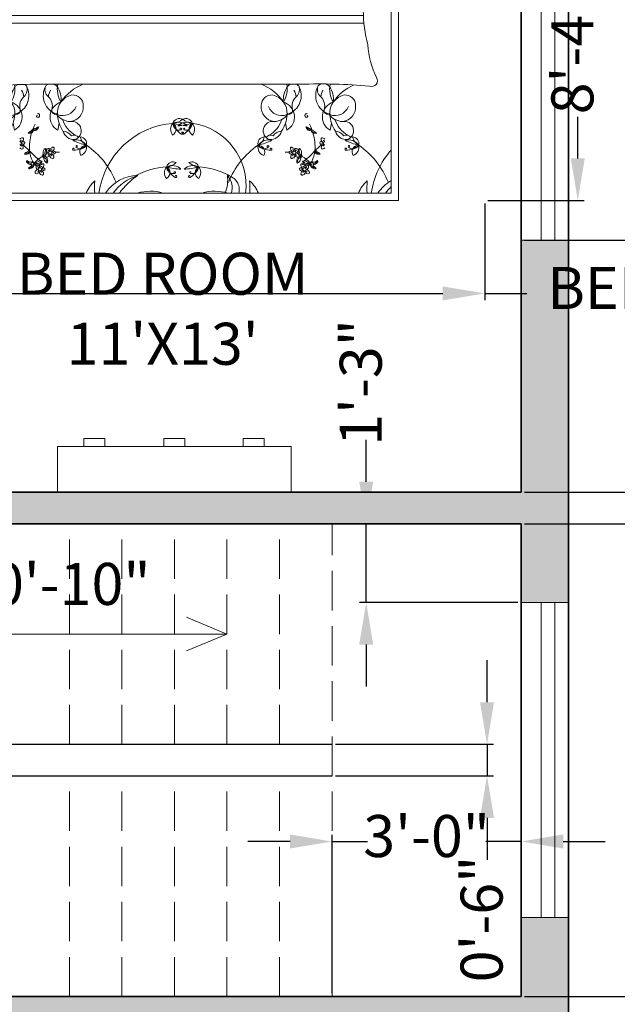
# Model space of a CAD drawing. Units: inches. Extents: x 2073 to 2646, y 2372 to 3017.
# Tile 6 of 8: x 2428 to 2542, y 2686 to 2874. Entities that reach past the tile are written whole.
import ezdxf

# ---------------------------------------------------------------- set-up
doc = ezdxf.new("R2010")
doc.units = ezdxf.units.IN
doc.linetypes.add('DASH', pattern=[0.35, 0.25, -0.1])
for name, color, linetype, lineweight in [('A-ANNO-DIMS', 2, 'Continuous', 18), ('A-ANNO-SYMB', 7, 'Continuous', 18), ('A-AREA-IDEN', 7, 'Continuous', 25), ('A-FLOR-STRS', 7, 'Continuous', 25), ('A-FLOR-STRS-HIDN', 7, 'DASH', 18), ('A-FURN', 8, 'Continuous', 18), ('A-GLAZ', 4, 'Continuous', 18), ('A-WALL', 7, 'Continuous', 35), ('A-WALL-PATT', 30, 'Continuous', 13)]:
    doc.layers.add(name, color=color, linetype=linetype, lineweight=lineweight)
doc.styles.get("Standard").update_dxf_attribs({"font": 'arial.ttf'})
doc.dimstyles.new('ISO-25', dxfattribs={"dimtxt": 8, "dimasz": 8, "dimexe": 1.25, "dimexo": 0.625, "dimtad": 0, "dimdec": 1, "dimlunit": 4, "dimtxsty": 'Standard', "dimcen": 2.5, "dimadec": 0, "dimazin": 0, "dimtfac": 1, "dimtdec": 1, "dimtmove": 0, "dimatfit": 3, "dimfxl": 1, "dimarcsym": 0})

# ---------------------------------------------------------------- blocks, each defined once
blk = doc.blocks.new('bed')
at = {"color": 0}
for p, q in [((2249.53, 3172.75), (2367.64, 3172.75)), ((2273.15, 3172.75), (2273.15, 3140.33)), ((2261.34, 3155.19), (2261.34, 3170.62)), ((2344.02, 3171.23), (2273.15, 3171.23)), ((2355.83, 3155.19), (2355.83, 3170.62)), ((2269.06, 3162.9), (2253.62, 3162.9)), ((2348.11, 3162.9), (2363.55, 3162.9)), ((2273.15, 3154.08), (2344.02, 3154.08)), ((2289.56, 3150.57), (2302.44, 3154.08)), ((2305.6, 3154.08), (2299.13, 3145.07)), ((2280.95, 3147.46), (2289.56, 3150.57)), ((2343.7, 3149.18), (2301.65, 3148.59)), ((2276.4, 3144.12), (2280.95, 3147.46)), ((2343.66, 3147.96), (2300.77, 3147.36)), ((2272.09, 3139.1), (2276.4, 3144.12)), ((2299.13, 3145.07), (2296.5, 3138.14)), ((2343.59, 3144.24), (2298.75, 3144.07)), ((2343.6, 3143.03), (2298.28, 3142.85)), ((2273.05, 3138.14), (2272.09, 3139.1)), ((2277.84, 3138.62), (2273.05, 3138.14)), ((2283.82, 3138.14), (2277.84, 3138.62)), ((2289.08, 3137.42), (2283.82, 3138.14)), ((2296.5, 3138.14), (2296.02, 3135.03)), ((2292.19, 3135.99), (2289.08, 3137.42)), ((2296.02, 3135.03), (2292.19, 3135.99)), ((2265.12, 3114.85), (2271.8, 3114.85)), ((2265.12, 3072.3), (2265.12, 3114.85)), ((2344.68, 3114.85), (2351.23, 3114.85)), ((2351.23, 3114.85), (2351.23, 3072.3)), ((2271.8, 3113.48), (2266.49, 3113.48)), ((2266.49, 3113.48), (2266.49, 3073.67)), ((2349.86, 3113.48), (2344.65, 3113.48)), ((2349.86, 3073.67), (2349.86, 3113.48)), ((2344.56, 3107.48), (2271.79, 3107.48)), ((2344.67, 3106.01), (2271.79, 3106.01)), ((2332.56, 3094.41), (2284.61, 3094.41)), ((2278.13, 3085.65), (2277.87, 3086.98)), ((2286.38, 3085.65), (2286.64, 3086.98)), ((2329.96, 3085.65), (2329.7, 3086.98)), ((2338.22, 3085.65), (2338.48, 3086.98)), ((2266.49, 3073.67), (2349.86, 3073.67)), ((2351.23, 3072.3), (2265.12, 3072.3))]:
    blk.add_line(p, q, dxfattribs=at)
for points in [[(2273.15, 3153.06), (2249.53, 3153.06), (2249.53, 3172.75)], [(2344.02, 3172.75), (2344.02, 3153.06), (2367.64, 3153.06), (2367.64, 3172.75)], [(2261.34, 3162.9), (2262.72, 3165.29)], [(2355.83, 3162.9), (2354.45, 3165.29)], [(2261.34, 3162.9), (2262.72, 3160.52)], [(2355.83, 3162.9), (2354.45, 3160.52)]]:
    blk.add_lwpolyline(points, dxfattribs=at)
for points in [[(2279.94, 3169.8, 0.074897), (2280.08, 3162.09, -0.472817)], [(2337.23, 3169.8, -0.074897), (2337.09, 3162.09, 0.472817)], [(2308.03, 3161.66, 0.14099), (2308.27, 3169.53, 0.235245)], [(2313.08, 3161.66, -0.14099), (2312.84, 3169.53, -0.235245)], [(2271.85, 3128.28, 0.001242), (2271.79, 3105.87, -0.127202), (2269.42, 3094.7)], [(2344.52, 3108.41, 0.056112), (2345.38, 3101.91, 0.095341), (2347.04, 3095.66)]]:
    blk.add_lwpolyline(points, format="xyb", dxfattribs=at)
for centre, radius in [((2261.34, 3162.9), 5.51), ((2355.83, 3162.9), 5.51), ((2261.34, 3162.9), 2.76), ((2355.83, 3162.9), 2.76), ((2284.95, 3081.37), 0.301), ((2331.4, 3081.37), 0.301), ((2282.98, 3078.2), 0.301), ((2333.36, 3078.2), 0.301)]:
    blk.add_circle(centre, radius, dxfattribs=at)
for centre, radius, start, end in [((2345.04, 4293.82), 1125.9, 266.68521, 267.14978), ((2296.12, 3127.06), 42.84, 82.2196, 99.497), ((2323.22, 3149.14), 20.76, 76.3427, 101.1841), ((2272.13, 4293.82), 1125.9, 272.85022, 273.31479), ((2305.17, 3148.71), 21.05, 81.5249, 103.96), ((2314.46, 3163.91), 5.84, 63.3437, 106.1026), ((2294.98, 3158.99), 15.22, 155.1316, 191.7583), ((2322.19, 3158.99), 15.22, 348.2417, 24.8684), ((2294.11, 3157.71), 14.47, 354.0129, 15.8293), ((2327, 3157.71), 14.47, 164.1707, 185.9871), ((2284.15, 3171.19), 15.83, 255.1039, 281.0369), ((2292.48, 3182.44), 27.45, 258.0397, 289.2615), ((2303.6, 3176.44), 20.83, 259.8617, 283.6238), ((2315.25, 3161.88), 6.26, 245.0183, 288.5407), ((2326.19, 3170.02), 15.03, 243.8761, 286.1746), ((2333.02, 3171.19), 15.83, 258.9631, 284.8961), ((2555.75, 3139.65), 212.22, 176.1, 180.9282), ((2163.8, 3136.16), 108.33, 355.8294, 1.553), ((2274.12, 3180.92), 44.58, 267.4519, 281.3392), ((2284.77, 3127.79), 9.61, 66.2616, 101.3392), ((2304.22, 3179.66), 45.8, 250.1194, 259.3383), ((2620.36, 3131.93), 276.84, 179.1145, 184.8735), ((2295.75, 3134.94), 0.285, 268.8623, 19.7536), ((2346.15, 3095.06), 1.08, 246.5219, 33.8264), ((2270.51, 3094.78), 1.09, 183.98, 297.3412), ((2283.2, 2971.46), 122.95, 89.3433, 95.6887), ((2270.05, 3086.09), 8.94, 33.6671, 63.2997), ((2282.03, 3091.41), 4.56, 145.785, 184.7304), ((2273.33, 3093.53), 4.89, 328.8218, 9.1554), ((2279.39, 3093.1), 1.42, 120.0293, 142.325), ((2277.12, 3092.26), 3.76, 289.2822, 29.1751), ((2276.55, 3091.58), 3.4, 7.436, 29.9149), ((2278.79, 3093.38), 1.77, 311.5653, 23.8354), ((2279.39, 3093.1), 1.42, 44.4517, 63.558), ((2287.39, 3092.26), 3.76, 150.8249, 250.7178), ((2285.72, 3093.38), 1.77, 156.1646, 228.4347), ((2285.12, 3093.1), 1.42, 113.229, 135.5483), ((2287.96, 3091.58), 3.4, 150.0851, 172.564), ((2285.12, 3093.1), 1.42, 37.675, 66.7144), ((2282.48, 3091.41), 4.56, 355.2696, 34.215), ((2291.18, 3093.53), 4.89, 169.7133, 211.1782), ((2294.46, 3086.09), 8.94, 111.4941, 146.3329), ((2321.89, 3086.09), 8.94, 33.6671, 68.5059), ((2333.87, 3091.41), 4.56, 145.785, 184.7304), ((2325.17, 3093.53), 4.89, 328.8218, 10.2867), ((2331.23, 3093.1), 1.42, 113.2856, 142.325), ((2328.96, 3092.26), 3.76, 289.2822, 29.1751), ((2328.39, 3091.58), 3.4, 7.436, 29.9149), ((2331.23, 3093.1), 1.42, 44.4517, 66.7144), ((2330.63, 3093.38), 1.77, 311.5653, 23.8354), ((2336.18, 2979.53), 114.93, 85.2402, 91.8035), ((2339.23, 3092.26), 3.76, 150.8249, 250.7178), ((2337.56, 3093.38), 1.77, 156.1646, 228.4347), ((2336.96, 3093.1), 1.42, 106.6343, 135.5483), ((2339.8, 3091.58), 3.4, 150.0851, 172.564), ((2336.96, 3093.1), 1.42, 37.675, 72.5814), ((2334.32, 3091.41), 4.56, 355.2696, 34.215), ((2343.02, 3093.53), 4.89, 169.249, 211.1782), ((2346.3, 3086.09), 8.94, 113.6453, 146.3329), ((2275.26, 3090.38), 1.99, 84.4856, 181.0538), ((2274.65, 3088.91), 3.55, 355.2933, 76.921), ((2281.57, 3090.25), 2.42, 131.5653, 195.1471), ((2282.94, 3090.25), 2.42, 344.8529, 48.4347), ((2289.86, 3088.91), 3.55, 103.079, 184.7067), ((2289.25, 3090.38), 1.99, 358.9462, 95.5144), ((2327.09, 3090.38), 1.99, 84.4856, 181.0538), ((2326.48, 3088.91), 3.55, 355.2933, 76.921), ((2333.4, 3090.25), 2.42, 131.5653, 195.1471), ((2334.78, 3090.25), 2.42, 344.8529, 48.4347), ((2341.7, 3088.91), 3.55, 103.079, 184.7067), ((2341.09, 3090.38), 1.99, 358.9462, 95.5144), ((2276.08, 3090.1), 2.82, 174.9449, 262.8857), ((2277.18, 3091.17), 2.74, 201.5819, 291.4221), ((2276.66, 3088.19), 2.94, 299.9085, 73.1337), ((2278.52, 3089.43), 0.733, 257.3041, 15.1471), ((2287.85, 3088.19), 2.94, 106.8663, 240.0915), ((2285.99, 3089.43), 0.733, 164.8529, 282.6959), ((2287.32, 3091.17), 2.74, 248.5779, 338.4181), ((2288.43, 3090.1), 2.82, 277.1143, 5.0551), ((2327.91, 3090.1), 2.82, 174.9449, 262.8857), ((2329.02, 3091.17), 2.74, 201.5819, 291.4221), ((2328.5, 3088.19), 2.94, 299.9085, 73.1337), ((2330.36, 3089.43), 0.733, 257.3041, 15.1471), ((2339.68, 3088.19), 2.94, 106.8663, 240.0915), ((2337.82, 3089.43), 0.733, 164.8529, 282.6959), ((2339.16, 3091.17), 2.74, 248.5779, 338.4181), ((2340.27, 3090.1), 2.82, 277.1143, 5.0551), ((2275.43, 3085.55), 1.77, 80.264, 250.8688), ((2271.91, 3089.45), 5.58, 301.2614, 341.7045), ((2275.58, 3090.72), 3.43, 272.3591, 324.0401), ((2271.86, 3089), 6.34, 326.2883, 356.5076), ((2282.03, 3091.41), 4.56, 212.7011, 216.3445), ((2282.59, 3088.31), 0.228, 102.7051, 280.4384), ((2282.57, 3088.45), 0.37, 280.4384, 100.4136), ((2282.48, 3091.41), 4.56, 323.6555, 327.2989), ((2288.92, 3090.72), 3.43, 215.9599, 267.6409), ((2292.65, 3089), 6.34, 183.4924, 213.7117), ((2292.6, 3089.45), 5.58, 198.2955, 238.7386), ((2289.08, 3085.55), 1.77, 289.1312, 99.736), ((2309.53, 3086.61), 1.28, 63.0274, 163.8037), ((2308.24, 3089.6), 2.63, 271.4585, 315.3727), ((2310.75, 3086.61), 1.28, 16.1963, 116.9726), ((2312.05, 3089.6), 2.63, 224.6273, 268.5415), ((2327.26, 3085.55), 1.77, 80.264, 250.8688), ((2323.75, 3089.45), 5.58, 301.2614, 341.7045), ((2327.42, 3090.72), 3.43, 272.3591, 324.0401), ((2323.7, 3089), 6.34, 326.2883, 356.5076), ((2333.87, 3091.41), 4.56, 212.7011, 216.3445), ((2333.78, 3088.45), 0.37, 79.5864, 259.5616), ((2333.75, 3088.31), 0.228, 259.5616, 77.2949), ((2334.32, 3091.41), 4.56, 323.6555, 327.2989), ((2340.76, 3090.72), 3.43, 215.9599, 267.6409), ((2344.49, 3089), 6.34, 183.4924, 213.7117), ((2344.44, 3089.45), 5.58, 198.2955, 238.7386), ((2340.92, 3085.55), 1.77, 289.1312, 99.736), ((2275, 3086.08), 2.21, 265.969, 344.3045), ((2277.38, 3083.14), 2.36, 96.1662, 141.5825), ((2279.99, 3086.89), 1.9, 308.2101, 316.3071), ((2281.16, 3085.65), 0.567, 278.3432, 4.2869), ((2280.84, 3086.14), 0.99, 300.656, 332.6341), ((2281.59, 3085.49), 0.241, 55.7657, 157.4417), ((2290.78, 3082.37), 9.78, 153.0032, 159.8941), ((2281.96, 3085.71), 0.241, 84.3784, 186.0543), ((2281.74, 3086.68), 0.99, 269.1859, 301.164), ((2282.03, 3086.17), 0.567, 237.5332, 323.4768), ((2281.48, 3087.78), 1.9, 285.5129, 293.6099), ((2282.72, 3085.65), 0.62, 87.3579, 140.4944), ((2281.28, 3087.43), 1.87, 301.164, 321.5612), ((2279.77, 3087.76), 3.33, 324.6898, 333.4936), ((2287.12, 3083.14), 2.36, 38.4175, 83.8338), ((2289.51, 3086.08), 2.21, 195.6955, 274.031), ((2309.5, 3071.59), 15.42, 94.4623, 172.255), ((2309.57, 3085.82), 1.71, 137.7873, 219.1145), ((2307.63, 3085.87), 1.29, 298.5391, 58.3627), ((2309.31, 3084.75), 2.44, 45.5411, 114.3101), ((2311.53, 3097.27), 10.79, 252.593, 267.2582), ((2309.56, 3086.92), 1.26, 177.7585, 283.852), ((2311.99, 3088.23), 3.9, 198.9159, 238.011), ((2310.98, 3084.75), 2.44, 65.6899, 134.4589), ((2308.75, 3097.27), 10.79, 272.7418, 287.407), ((2309.83, 3085.86), 0.167, 283.852, 219.9245), ((2310.44, 3085.92), 0.101, 320.1909, 256.0209), ((2308.29, 3088.23), 3.9, 301.989, 341.0841), ((2310.72, 3086.92), 1.26, 256.148, 2.2415), ((2312.66, 3085.87), 1.29, 121.6373, 241.4609), ((2310.71, 3085.82), 1.71, 320.8855, 42.2127), ((2310.28, 3075.15), 11.94, 352.8636, 81.8197), ((2326.84, 3086.08), 2.21, 265.969, 344.3045), ((2329.22, 3083.14), 2.36, 96.1662, 141.5825), ((2335.06, 3087.43), 1.87, 218.4388, 238.836), ((2333.63, 3085.65), 0.62, 39.5056, 92.6421), ((2336.58, 3087.76), 3.33, 206.5064, 215.3102), ((2334.32, 3086.17), 0.567, 216.5232, 302.4668), ((2334.61, 3086.68), 0.99, 238.836, 270.8141), ((2334.87, 3087.78), 1.9, 246.3901, 254.4871), ((2325.57, 3082.37), 9.78, 20.1059, 26.9968), ((2334.38, 3085.71), 0.241, 353.9457, 95.6216), ((2334.76, 3085.49), 0.241, 22.5583, 124.2343), ((2335.19, 3085.65), 0.567, 175.7131, 261.6568), ((2335.5, 3086.14), 0.99, 207.3659, 239.344), ((2336.35, 3086.89), 1.9, 223.6929, 231.7899), ((2341.35, 3086.08), 2.21, 195.6955, 274.031), ((2338.96, 3083.14), 2.36, 38.4175, 83.8338), ((2273.92, 3083.1), 1.28, 92.9516, 193.728), ((2271.31, 3085.04), 2.63, 301.3827, 345.2969), ((2274.66, 3081.37), 2.44, 75.4653, 144.2343), ((2270.34, 3093.33), 10.79, 282.5173, 297.1824), ((2275.06, 3083.63), 1.09, 63.9755, 143.2681), ((2279.54, 3083.62), 0.502, 101.5637, 142.6358), ((2279.47, 3083.44), 0.287, 91.1081, 181.8675), ((2279.13, 3084.01), 0.723, 288.7263, 352.5032), ((2279.63, 3083.98), 0.232, 345.2356, 144.9248), ((2281.29, 3084.79), 0.62, 101.3256, 154.4621), ((2280.4, 3086.9), 1.87, 280.2588, 300.656), ((2280.83, 3088.39), 3.33, 268.3264, 277.1302), ((2290.78, 3082.37), 9.78, 163.5842, 183.8277), ((2289.45, 3083.63), 1.09, 36.7319, 116.0245), ((2289.85, 3081.37), 2.44, 35.7657, 104.5347), ((2294.17, 3093.33), 10.79, 242.8176, 257.4827), ((2290.59, 3083.1), 1.28, 346.272, 87.0484), ((2293.2, 3085.04), 2.63, 194.7031, 238.6173), ((2310.03, 3085.09), 0.192, 238.011, 71.5592), ((2310.06, 3085.18), 0.093, 71.5592, 188.0167), ((2310.25, 3085.09), 0.192, 108.4408, 301.989), ((2310.22, 3085.18), 0.093, 351.9833, 108.4408), ((2325.76, 3083.1), 1.28, 92.9516, 193.728), ((2323.15, 3085.04), 2.63, 301.3827, 345.2969), ((2326.5, 3081.37), 2.44, 75.4653, 144.2343), ((2322.18, 3093.33), 10.79, 282.5173, 297.1824), ((2326.9, 3083.63), 1.09, 63.9755, 143.2681), ((2325.57, 3082.37), 9.78, 356.1723, 16.4158), ((2335.95, 3086.9), 1.87, 239.344, 259.7412), ((2335.52, 3088.39), 3.33, 262.8698, 271.6736), ((2335.06, 3084.79), 0.62, 25.5379, 78.6744), ((2336.72, 3083.98), 0.232, 35.0752, 194.7644), ((2337.21, 3084.01), 0.723, 187.4968, 251.2737), ((2336.88, 3083.44), 0.287, 358.1325, 88.8919), ((2336.81, 3083.62), 0.502, 37.3642, 78.4363), ((2341.29, 3083.63), 1.09, 36.7319, 116.0245), ((2341.69, 3081.37), 2.44, 35.7657, 104.5347), ((2346, 3093.33), 10.79, 242.8176, 257.4827), ((2345.04, 3085.04), 2.63, 194.7031, 238.6173), ((2342.42, 3083.1), 1.28, 346.272, 87.0484), ((2255.01, 3071.59), 15.42, 7.745, 41.8856), ((2281.39, 3070.07), 15.42, 124.3865, 158.5908), ((2274.35, 3082.43), 1.71, 167.7115, 249.0387), ((2272.64, 3081.51), 1.29, 328.4633, 88.2869), ((2275.25, 3085.73), 3.9, 228.8402, 267.9352), ((2273.8, 3083.38), 1.26, 207.6827, 313.7762), ((2274.56, 3082.59), 0.167, 313.7762, 249.7183), ((2275.1, 3082.12), 0.093, 101.4834, 217.9409), ((2275.12, 3082.03), 0.192, 267.9352, 101.4834), ((2279.12, 3083.15), 0.301, 273.2768, 86.7232), ((2279.53, 3082.6), 0.497, 217.7621, 259.0403), ((2280.07, 3083.26), 0.913, 203.4276, 227.6104), ((2279.78, 3082.86), 0.622, 80.3487, 133.6538), ((2279.66, 3083.37), 0.492, 229.7889, 317.6792), ((2279.11, 3082.33), 0.699, 355.053, 68.3618), ((2279.66, 3082.21), 0.985, 83.0852, 105.7171), ((2279.58, 3082.29), 0.231, 232.4737, 355.053), ((2272.84, 3074.04), 11.21, 43.1541, 52.0459), ((2279.84, 3083.22), 0.259, 317.6792, 80.3487), ((2280.45, 3081.67), 0.567, 278.3432, 4.2869), ((2280.14, 3082.17), 0.99, 300.656, 332.6341), ((2280.88, 3081.52), 0.241, 55.7657, 157.4417), ((2285.91, 3082.12), 4.9, 184.756, 209.2041), ((2292.97, 3092.56), 16.14, 222.2412, 232.1744), ((2282.65, 3081.81), 1.37, 304.5369, 16.3699), ((2284.55, 3081.43), 0.97, 127.3105, 187.9252), ((2283.22, 3081.54), 0.996, 355.0106, 41.658), ((2284.62, 3081.78), 0.41, 126.1046, 271.4281), ((2284.57, 3081.9), 0.295, 353.7526, 131.7054), ((2284.3, 3081.55), 0.414, 0.0645, 61.1507), ((2284.39, 3081.9), 0.473, 311.8413, 355.7877), ((2285.37, 3081.83), 0.502, 101.5637, 176.365), ((2285.3, 3081.65), 0.287, 91.1081, 181.8675), ((2285.61, 3081.07), 0.622, 80.3487, 133.6538), ((2284.96, 3082.22), 0.723, 288.7263, 352.5032), ((2285.46, 3082.19), 0.232, 345.2356, 144.9248), ((2285.67, 3081.43), 0.259, 317.6792, 80.3487), ((2289.39, 3082.03), 0.192, 78.5166, 272.0648), ((2289.26, 3085.73), 3.9, 272.0648, 311.1598), ((2289.41, 3082.12), 0.093, 322.0591, 78.5166), ((2290.71, 3083.38), 1.26, 226.2238, 332.3173), ((2289.97, 3082.66), 0.101, 290.2667, 226.2271), ((2291.87, 3081.51), 1.29, 91.7131, 211.5367), ((2290.16, 3082.43), 1.71, 290.9613, 12.2885), ((2283.12, 3070.07), 15.42, 21.4092, 55.6135), ((2333.23, 3070.07), 15.42, 124.3865, 158.5908), ((2326.19, 3082.43), 1.71, 167.7115, 249.0387), ((2325.64, 3083.38), 1.26, 207.6827, 313.7762), ((2327.09, 3085.73), 3.9, 228.8402, 267.9352), ((2324.48, 3081.51), 1.29, 328.4633, 88.2869), ((2326.39, 3082.59), 0.167, 313.7762, 249.7183), ((2326.93, 3082.12), 0.093, 101.4834, 217.9409), ((2326.95, 3082.03), 0.192, 267.9352, 101.4834), ((2330.68, 3081.43), 0.259, 99.6513, 222.3208), ((2330.74, 3081.07), 0.622, 46.3462, 99.6513), ((2330.89, 3082.19), 0.232, 35.0752, 194.7644), ((2331.38, 3082.22), 0.723, 187.4968, 251.2737), ((2331.05, 3081.65), 0.287, 358.1325, 88.8919), ((2330.98, 3081.83), 0.502, 3.635, 78.4363), ((2331.77, 3081.9), 0.295, 48.2946, 186.2474), ((2331.95, 3081.9), 0.473, 184.2123, 228.1587), ((2332.05, 3081.55), 0.414, 118.8493, 179.9355), ((2331.73, 3081.78), 0.41, 268.5719, 53.8954), ((2333.13, 3081.54), 0.996, 138.342, 184.9894), ((2333.7, 3081.81), 1.37, 163.6301, 235.4631), ((2331.79, 3081.43), 0.97, 352.0748, 52.6895), ((2323.38, 3092.56), 16.14, 307.8256, 317.7588), ((2330.44, 3082.12), 4.9, 330.7959, 355.244), ((2343.51, 3074.04), 11.21, 127.9541, 136.8459), ((2335.46, 3081.52), 0.241, 22.5583, 124.2343), ((2335.89, 3081.67), 0.567, 175.7131, 261.6568), ((2336.21, 3082.17), 0.99, 207.3659, 239.344), ((2336.51, 3083.22), 0.259, 99.6513, 222.3208), ((2336.68, 3083.37), 0.492, 222.3208, 310.2111), ((2336.57, 3082.86), 0.622, 46.3462, 99.6513), ((2337.24, 3082.33), 0.699, 111.6382, 184.947), ((2336.77, 3082.29), 0.231, 184.947, 307.5263), ((2336.69, 3082.21), 0.985, 74.2829, 96.9148), ((2336.28, 3083.26), 0.913, 312.3896, 336.5724), ((2336.82, 3082.6), 0.497, 280.9597, 322.2379), ((2337.23, 3083.15), 0.301, 93.2768, 266.7232), ((2341.23, 3082.03), 0.192, 78.5166, 272.0648), ((2341.1, 3085.73), 3.9, 272.0648, 311.1598), ((2341.25, 3082.12), 0.093, 322.0591, 78.5166), ((2342.55, 3083.38), 1.26, 226.2238, 332.3173), ((2341.81, 3082.66), 0.101, 290.2667, 226.2271), ((2343.7, 3081.51), 1.29, 91.7131, 211.5367), ((2341.99, 3082.43), 1.71, 290.9613, 12.2885), ((2334.95, 3070.07), 15.42, 21.4092, 55.6135), ((2361.34, 3071.59), 15.42, 138.1144, 172.255), ((2280.59, 3080.82), 0.62, 101.3256, 154.4621), ((2279.69, 3082.92), 1.87, 280.2588, 300.656), ((2280.12, 3084.42), 3.33, 268.3264, 277.1302), ((2279.29, 3082.92), 1.9, 308.2101, 316.3071), ((2280.79, 3079.73), 0.336, 146.8636, 236.9021), ((2285.53, 3087.13), 8.79, 235.1882, 238.8844), ((2281.37, 3080.22), 0.909, 199.4799, 267.6828), ((2286.41, 3075.61), 5.88, 120.544, 139.818), ((2283.06, 3078.85), 0.97, 70.0041, 130.6188), ((2283.38, 3081.51), 0.833, 272.8499, 356.1226), ((2282.79, 3081.18), 0.807, 321.7607, 7.9252), ((2282.96, 3080.02), 0.807, 8.7227, 54.8872), ((2283, 3079.38), 1.37, 0.278, 72.111), ((2283.62, 3079.88), 0.833, 20.5253, 88.5375), ((2284.72, 3080.29), 0.97, 188.7227, 249.3375), ((2284.32, 3080.8), 0.298, 148.0499, 225.6268), ((2286.41, 3075.61), 5.88, 113.0501, 113.8477), ((2284.87, 3080.46), 0.948, 104.7558, 148.0499), ((2284.34, 3081.14), 0.594, 247.4086, 351.4386), ((2283.47, 3079.81), 0.996, 334.9899, 21.6373), ((2284.51, 3081.11), 0.199, 262.906, 7.132), ((2285.36, 3080.81), 0.497, 151.2196, 259.0403), ((2285.9, 3081.47), 0.913, 203.4276, 227.6104), ((2285.5, 3081.59), 0.492, 229.7889, 317.6792), ((2284.94, 3080.54), 0.699, 355.053, 68.3618), ((2285.49, 3080.43), 0.985, 83.0852, 105.7171), ((2285.41, 3080.5), 0.231, 232.4737, 355.053), ((2286.41, 3075.61), 5.88, 87.1071, 94.7585), ((2329.94, 3075.61), 5.88, 85.2415, 92.8929), ((2330.85, 3081.59), 0.492, 222.3208, 310.2111), ((2331.41, 3080.54), 0.699, 111.6382, 184.947), ((2330.94, 3080.5), 0.231, 184.947, 307.5263), ((2330.86, 3080.43), 0.985, 74.2829, 96.9148), ((2330.45, 3081.47), 0.913, 312.3896, 336.5724), ((2330.99, 3080.81), 0.497, 280.9597, 28.7804), ((2332.01, 3081.14), 0.594, 188.5614, 292.5914), ((2331.84, 3081.11), 0.199, 172.868, 277.094), ((2331.48, 3080.46), 0.948, 31.9501, 75.2442), ((2332.87, 3079.81), 0.996, 158.3627, 205.0101), ((2332.73, 3079.88), 0.833, 91.4625, 159.4747), ((2333.34, 3079.38), 1.37, 107.889, 179.722), ((2331.63, 3080.29), 0.97, 290.6625, 351.2773), ((2332.97, 3081.51), 0.833, 183.8774, 267.1501), ((2329.94, 3075.61), 5.88, 66.1523, 66.9499), ((2332.03, 3080.8), 0.298, 314.3732, 31.9501), ((2333.39, 3080.02), 0.807, 125.1128, 171.2773), ((2333.55, 3081.18), 0.807, 172.0748, 218.2393), ((2329.94, 3075.61), 5.88, 40.182, 59.456), ((2333.29, 3078.85), 0.97, 49.3812, 109.9959), ((2334.98, 3080.22), 0.909, 272.3172, 340.5201), ((2330.82, 3087.13), 8.79, 301.1156, 304.8118), ((2337.06, 3082.92), 1.9, 223.6929, 231.7899), ((2336.65, 3082.92), 1.87, 239.344, 259.7412), ((2335.55, 3079.73), 0.336, 303.0979, 33.1364), ((2336.22, 3084.42), 3.33, 262.8698, 271.6736), ((2335.76, 3080.82), 0.62, 25.5379, 78.6744), ((2281.27, 3079.88), 0.783, 212.8155, 277.3992), ((2280.81, 3079.35), 0.909, 266.9701, 338.2913), ((2276.02, 3085.84), 8.79, 302.6784, 306.3746), ((2281.04, 3078.63), 0.336, 214.3538, 304.3923), ((2281.17, 3079.91), 0.348, 238.8844, 314.2646), ((2281.09, 3079.13), 0.783, 280.3057, 17.1958), ((2281.03, 3079.05), 0.348, 306.3746, 21.7548), ((2281.59, 3079.27), 0.262, 19.3605, 201.7548), ((2281.59, 3079.47), 0.262, 311.8703, 134.2646), ((2286.53, 3077.08), 5.24, 153.7819, 158.2913), ((2282.36, 3080.66), 1.37, 247.2305, 319.0635), ((2281.9, 3080.2), 0.807, 264.4544, 310.6188), ((2285.91, 3082.12), 4.9, 214.0033, 222.4917), ((2282.49, 3079.88), 0.833, 218.3208, 298.8162), ((2282.9, 3077.29), 0.948, 104.7558, 148.0499), ((2282.65, 3078.61), 0.41, 126.1046, 271.4281), ((2282.61, 3078.72), 0.295, 353.7526, 131.7054), ((2282.54, 3077.94), 0.199, 262.906, 7.132), ((2282.33, 3078.37), 0.414, 0.0645, 61.1507), ((2282.43, 3078.73), 0.473, 311.8413, 355.7877), ((2282.43, 3080.03), 0.996, 297.7043, 344.3516), ((2283.4, 3078.66), 0.502, 101.5637, 176.365), ((2283.33, 3078.48), 0.287, 91.1081, 181.8675), ((2283.93, 3078.3), 0.913, 203.4276, 227.6104), ((2283.64, 3077.9), 0.622, 80.3487, 133.6538), ((2283.53, 3078.42), 0.492, 229.7889, 317.6792), ((2283, 3079.05), 0.723, 288.7263, 352.5032), ((2282.97, 3077.37), 0.699, 355.053, 68.3618), ((2283.52, 3077.26), 0.985, 83.0852, 105.7171), ((2283.49, 3079.02), 0.232, 345.2356, 144.9248), ((2283.7, 3078.26), 0.259, 317.6792, 80.3487), ((2308.32, 3063.33), 15.42, 94.4623, 117.4146), ((2308.39, 3077.56), 1.71, 137.7873, 219.1145), ((2306.45, 3077.61), 1.29, 298.5391, 58.3627), ((2308.35, 3078.35), 1.28, 63.0274, 163.8037), ((2307.06, 3081.34), 2.63, 271.4585, 315.3727), ((2308.13, 3076.49), 2.44, 45.5411, 114.3101), ((2310.81, 3079.97), 3.9, 198.9159, 238.011), ((2310.35, 3089), 10.79, 252.593, 267.2582), ((2308.38, 3078.66), 1.26, 177.7585, 283.852), ((2312.16, 3076.49), 2.44, 65.6899, 134.4589), ((2309.93, 3089), 10.79, 272.7418, 287.407), ((2311.93, 3078.35), 1.28, 16.1963, 116.9726), ((2313.23, 3081.34), 2.63, 224.6273, 268.5415), ((2309.47, 3079.97), 3.9, 301.989, 341.0841), ((2311.9, 3078.66), 1.26, 256.148, 2.2415), ((2313.84, 3077.61), 1.29, 121.6373, 241.4609), ((2311.89, 3077.56), 1.71, 320.8855, 42.2127), ((2311.96, 3063.33), 15.42, 62.5854, 85.5377), ((2332.65, 3078.26), 0.259, 99.6513, 222.3208), ((2332.82, 3078.42), 0.492, 222.3208, 310.2111), ((2332.71, 3077.9), 0.622, 46.3462, 99.6513), ((2332.86, 3079.02), 0.232, 35.0752, 194.7644), ((2333.35, 3079.05), 0.723, 187.4968, 251.2737), ((2333.37, 3077.37), 0.699, 111.6382, 184.947), ((2332.83, 3077.26), 0.985, 74.2829, 96.9148), ((2333.99, 3080.66), 1.37, 220.9365, 292.7695), ((2333.91, 3080.03), 0.996, 195.6484, 242.2957), ((2333.01, 3078.48), 0.287, 358.1325, 88.8919), ((2332.42, 3078.3), 0.913, 312.3896, 336.5724), ((2332.95, 3078.66), 0.502, 3.635, 78.4363), ((2333.85, 3079.88), 0.833, 241.1838, 321.6792), ((2333.74, 3078.72), 0.295, 48.2946, 186.2474), ((2333.92, 3078.73), 0.473, 184.2123, 228.1587), ((2334.02, 3078.37), 0.414, 118.8493, 179.9355), ((2333.81, 3077.94), 0.199, 172.868, 277.094), ((2333.7, 3078.61), 0.41, 268.5719, 53.8954), ((2333.44, 3077.29), 0.948, 31.9501, 75.2442), ((2334.44, 3080.2), 0.807, 229.3812, 275.5456), ((2330.44, 3082.12), 4.9, 317.5083, 325.9967), ((2335.25, 3079.13), 0.783, 162.8042, 259.6943), ((2334.75, 3079.47), 0.262, 45.7354, 228.1297), ((2334.75, 3079.27), 0.262, 338.2452, 160.6395), ((2329.82, 3077.08), 5.24, 21.7087, 26.2181), ((2335.53, 3079.35), 0.909, 201.7087, 273.0299), ((2335.18, 3079.91), 0.348, 225.7354, 301.1156), ((2335.32, 3079.05), 0.348, 158.2452, 233.6254), ((2335.08, 3079.88), 0.783, 262.6008, 327.1845), ((2340.32, 3085.84), 8.79, 233.6254, 237.3216), ((2335.3, 3078.63), 0.336, 235.6077, 325.6462), ((2282.35, 3077.63), 0.298, 148.0499, 225.6268), ((2282.37, 3077.97), 0.594, 247.4086, 351.4386), ((2283.39, 3077.64), 0.497, 151.2196, 259.0403), ((2283.44, 3077.33), 0.231, 232.4737, 355.053), ((2301.77, 3069.53), 7.52, 91.272, 146.5383), ((2304.47, 3068.13), 9.37, 107.8504, 143.6964), ((2309.39, 3065.49), 13.93, 124.0123, 144.053), ((2308.65, 3077.6), 0.167, 283.852, 219.9245), ((2308.85, 3076.83), 0.192, 238.011, 71.5592), ((2308.88, 3076.92), 0.093, 71.5592, 188.0167), ((2311.44, 3076.83), 0.192, 108.4408, 301.989), ((2311.4, 3076.92), 0.093, 351.9833, 108.4408), ((2311.62, 3077.66), 0.101, 320.1909, 256.0209), ((2311.82, 3076.24), 6.91, 338.117, 6.6195), ((2318.16, 3074.32), 2.77, 346.3898, 79.0739), ((2316.08, 3074.7), 3.5, 342.8609, 41.9049), ((2332.91, 3077.33), 0.231, 184.947, 307.5263), ((2332.95, 3077.64), 0.497, 280.9597, 28.7804), ((2333.98, 3077.97), 0.594, 188.5614, 292.5914), ((2334, 3077.63), 0.298, 314.3732, 31.9501), ((2262.74, 3069.53), 7.52, 33.4617, 60.1116), ((2260.04, 3068.13), 9.37, 36.3036, 46.4814), ((2266.95, 3071.27), 6.27, 22.5547, 48.9546), ((2249.77, 3074.64), 21.34, 357.4081, 3.6519), ((2297.56, 3071.27), 6.27, 131.0454, 157.4453), ((2314.73, 3074.64), 21.34, 176.3481, 182.5919), ((2301.61, 3074.64), 21.34, 357.4081, 3.6519), ((2318.79, 3071.27), 6.27, 22.5547, 48.9546), ((2349.39, 3071.27), 6.27, 131.0454, 157.4453), ((2366.57, 3074.64), 21.34, 176.3481, 182.5919), ((2353.6, 3069.53), 7.52, 119.8884, 146.5383), ((2356.31, 3068.13), 9.37, 133.5186, 143.6964), ((2304.01, 3065.56), 8.48, 73.5431, 107.0202), ((2307.37, 3061.19), 12.54, 94.3787, 95.6357), ((2313.97, 3052.6), 22.41, 109.7217, 109.9028), ((2316.27, 3065.56), 8.48, 72.9798, 106.4569), ((2312.91, 3061.19), 12.54, 84.3643, 85.6213), ((2306.31, 3052.6), 22.41, 70.0972, 70.2783)]:
    blk.add_arc(centre, radius, start, end, dxfattribs=at)
blk = doc.blocks.new('GLAZ-60IN')
for p, q in [((0, 60), (0, 0)), ((2.6, 60), (2.6, 0))]:
    blk.add_line(p, q)
blk = doc.blocks.new('WALL-CONSOLE-44IN')
for points in [[(10.22, 44.47), (1.5, 44.47), (1.5, 0), (10.22, 0)], [(1.5, 39.34), (0, 39.34), (0, 35.33), (1.5, 35.33)], [(1.5, 24.24), (0, 24.24), (0, 20.23), (1.5, 20.23)], [(1.5, 8.99), (0, 8.99), (0, 4.98), (1.5, 4.98)]]:
    blk.add_lwpolyline(points, close=True)
blk = doc.blocks.new('*D35')
at = {"layer": 'A-ANNO-DIMS', "color": 0, "lineweight": -2, "transparency": 16777216}
for p, q in [((2398.23, 2838.6), (2398.23, 2820.25)), ((2516.35, 2838.6), (2516.35, 2820.25)), ((2406.23, 2821.5), (2508.35, 2821.5)), ((2516.35, 2821.5), (2524.35, 2821.5))]:
    blk.add_line(p, q, dxfattribs=at)
at = {"layer": 'A-ANNO-DIMS', "color": 0, "transparency": 16777216}
for points in [[(2406.23, 2822.84), (2406.23, 2820.17), (2398.23, 2821.5)], [(2508.35, 2822.84), (2508.35, 2820.17), (2516.35, 2821.5)]]:
    blk.add_solid(points, dxfattribs=at)
at = {"layer": 'Defpoints', "color": 0, "transparency": 16777216}
for p in [(2398.23, 2839.22), (2516.35, 2839.22), (2516.35, 2821.5)]:
    blk.add_point(p, dxfattribs=at)
at = {"layer": 'A-ANNO-DIMS', "color": 0, "transparency": 16777216, "insert": (2587.37, 2821.5), "char_height": 8, "attachment_point": 5}
blk.add_mtext('BED GROUP 9\'-10" TYP.', dxfattribs=at)
blk = doc.blocks.new('*D36')
at = {"layer": 'A-ANNO-DIMS', "color": 0, "lineweight": -2, "transparency": 16777216}
for p, q in [((2516.97, 2939.66), (2535.31, 2939.66)), ((2534.06, 2931.66), (2534.06, 2923.78)), ((2534.06, 2847.22), (2534.06, 2855.11)), ((2516.97, 2839.22), (2535.31, 2839.22))]:
    blk.add_line(p, q, dxfattribs=at)
at = {"layer": 'A-ANNO-DIMS', "color": 0, "transparency": 16777216}
for points in [[(2532.73, 2931.66), (2535.39, 2931.66), (2534.06, 2939.66)], [(2532.73, 2847.22), (2535.39, 2847.22), (2534.06, 2839.22)]]:
    blk.add_solid(points, dxfattribs=at)
at = {"layer": 'Defpoints', "color": 0, "transparency": 16777216}
for p in [(2516.35, 2939.66), (2534.06, 2939.66), (2516.35, 2839.22)]:
    blk.add_point(p, dxfattribs=at)
at = {"layer": 'A-ANNO-DIMS', "color": 0, "transparency": 16777216, "insert": (2534.06, 2889.44), "char_height": 8, "attachment_point": 5, "rotation": 90}
blk.add_mtext('8\'-4 1/2" TYP.', dxfattribs=at)
blk = doc.blocks.new('*D45')
at = {"layer": 'A-ANNO-DIMS', "color": 0, "lineweight": -2, "transparency": 16777216}
for p, q in [((2523.92, 2777.66), (2563.04, 2777.66)), ((2561.79, 2769.66), (2561.79, 2743.89)), ((2561.79, 2695.66), (2561.79, 2721.44)), ((2523.92, 2687.66), (2563.04, 2687.66))]:
    blk.add_line(p, q, dxfattribs=at)
at = {"layer": 'A-ANNO-DIMS', "color": 0, "transparency": 16777216}
for points in [[(2560.46, 2769.66), (2563.12, 2769.66), (2561.79, 2777.66)], [(2560.46, 2695.66), (2563.12, 2695.66), (2561.79, 2687.66)]]:
    blk.add_solid(points, dxfattribs=at)
at = {"layer": 'Defpoints', "color": 0, "transparency": 16777216}
for p in [(2523.29, 2777.66), (2561.79, 2777.66), (2523.29, 2687.66)]:
    blk.add_point(p, dxfattribs=at)
at = {"layer": 'A-ANNO-DIMS', "color": 0, "transparency": 16777216, "insert": (2561.79, 2732.66), "char_height": 8, "attachment_point": 5, "rotation": 90}
blk.add_mtext('7\'-6"', dxfattribs=at)
blk = doc.blocks.new('*D54')
at = {"layer": 'A-ANNO-DIMS', "color": 0, "lineweight": -2, "transparency": 16777216}
for p, q in [((2487.29, 2688.29), (2487.29, 2718.41)), ((2523.29, 2688.29), (2523.29, 2718.41)), ((2479.29, 2717.16), (2471.29, 2717.16)), ((2487.29, 2717.16), (2494.03, 2717.16)), ((2523.29, 2717.16), (2516.55, 2717.16)), ((2531.29, 2717.16), (2539.29, 2717.16))]:
    blk.add_line(p, q, dxfattribs=at)
at = {"layer": 'A-ANNO-DIMS', "color": 0, "transparency": 16777216}
for points in [[(2479.29, 2718.5), (2479.29, 2715.83), (2487.29, 2717.16)], [(2531.29, 2718.5), (2531.29, 2715.83), (2523.29, 2717.16)]]:
    blk.add_solid(points, dxfattribs=at)
at = {"layer": 'Defpoints', "color": 0, "transparency": 16777216}
for p in [(2523.29, 2717.16), (2487.29, 2687.66), (2523.29, 2687.66)]:
    blk.add_point(p, dxfattribs=at)
at = {"layer": 'A-ANNO-DIMS', "color": 0, "transparency": 16777216, "insert": (2505.29, 2717.16), "char_height": 8, "attachment_point": 5}
blk.add_mtext('3\'-0"', dxfattribs=at)
blk = doc.blocks.new('*D56')
at = {"layer": 'A-ANNO-DIMS', "color": 0, "lineweight": -2, "transparency": 16777216}
for p, q in [((2523.92, 2831.66), (2563.04, 2831.66)), ((2561.79, 2823.66), (2561.79, 2819.08)), ((2561.79, 2791.66), (2561.79, 2796.25)), ((2523.92, 2783.66), (2563.04, 2783.66))]:
    blk.add_line(p, q, dxfattribs=at)
at = {"layer": 'A-ANNO-DIMS', "color": 0, "transparency": 16777216}
for points in [[(2560.46, 2823.66), (2563.12, 2823.66), (2561.79, 2831.66)], [(2560.46, 2791.66), (2563.12, 2791.66), (2561.79, 2783.66)]]:
    blk.add_solid(points, dxfattribs=at)
at = {"layer": 'Defpoints', "color": 0, "transparency": 16777216}
for p in [(2523.29, 2831.66), (2561.79, 2831.66), (2523.29, 2783.66)]:
    blk.add_point(p, dxfattribs=at)
at = {"layer": 'A-ANNO-DIMS', "color": 0, "transparency": 16777216, "insert": (2561.79, 2807.66), "char_height": 8, "attachment_point": 5, "rotation": 90}
blk.add_mtext('4\'-0"', dxfattribs=at)
blk = doc.blocks.new('*D58')
at = {"layer": 'A-ANNO-DIMS', "color": 0, "lineweight": -2, "transparency": 16777216}
for p, q in [((2493.79, 2785.66), (2493.79, 2793.66)), ((2522.67, 2777.66), (2492.54, 2777.66)), ((2493.79, 2762.66), (2493.79, 2777.66)), ((2522.67, 2762.66), (2492.54, 2762.66)), ((2493.79, 2754.66), (2493.79, 2746.66))]:
    blk.add_line(p, q, dxfattribs=at)
at = {"layer": 'A-ANNO-DIMS', "color": 0, "transparency": 16777216}
for points in [[(2492.46, 2785.66), (2495.12, 2785.66), (2493.79, 2777.66)], [(2492.46, 2754.66), (2495.12, 2754.66), (2493.79, 2762.66)]]:
    blk.add_solid(points, dxfattribs=at)
at = {"layer": 'Defpoints', "color": 0, "transparency": 16777216}
for p in [(2493.79, 2777.66), (2523.29, 2777.66), (2523.29, 2762.66)]:
    blk.add_point(p, dxfattribs=at)
at = {"layer": 'A-ANNO-DIMS', "color": 0, "transparency": 16777216, "insert": (2493.79, 2804.55), "char_height": 8, "attachment_point": 5, "rotation": 90}
blk.add_mtext('1\'-3"', dxfattribs=at)
blk = doc.blocks.new('*D67')
at = {"layer": 'A-ANNO-DIMS', "color": 0, "lineweight": -2, "transparency": 16777216}
for p, q in [((2389.29, 2765.16), (2381.29, 2765.16)), ((2397.29, 2736.29), (2397.29, 2766.41)), ((2397.29, 2765.16), (2407.29, 2765.16)), ((2407.29, 2736.29), (2407.29, 2766.41)), ((2415.29, 2765.16), (2423.29, 2765.16))]:
    blk.add_line(p, q, dxfattribs=at)
at = {"layer": 'A-ANNO-DIMS', "color": 0, "transparency": 16777216}
for points in [[(2389.29, 2766.5), (2389.29, 2763.83), (2397.29, 2765.16)], [(2415.29, 2766.5), (2415.29, 2763.83), (2407.29, 2765.16)]]:
    blk.add_solid(points, dxfattribs=at)
at = {"layer": 'Defpoints', "color": 0, "transparency": 16777216}
for p in [(2407.29, 2765.16), (2397.29, 2735.66), (2407.29, 2735.66)]:
    blk.add_point(p, dxfattribs=at)
at = {"layer": 'A-ANNO-DIMS', "color": 0, "transparency": 16777216, "insert": (2437.66, 2765.16), "char_height": 8, "attachment_point": 5}
blk.add_mtext('0\'-10"', dxfattribs=at)
blk = doc.blocks.new('*D68')
at = {"layer": 'A-ANNO-DIMS', "color": 0, "lineweight": -2, "transparency": 16777216}
for p, q in [((2516.79, 2743.66), (2516.79, 2751.66)), ((2487.92, 2735.66), (2518.04, 2735.66)), ((2516.79, 2735.66), (2516.79, 2729.66)), ((2487.92, 2729.66), (2518.04, 2729.66)), ((2516.79, 2721.66), (2516.79, 2713.66))]:
    blk.add_line(p, q, dxfattribs=at)
at = {"layer": 'A-ANNO-DIMS', "color": 0, "transparency": 16777216}
for points in [[(2515.46, 2743.66), (2518.12, 2743.66), (2516.79, 2735.66)], [(2515.46, 2721.66), (2518.12, 2721.66), (2516.79, 2729.66)]]:
    blk.add_solid(points, dxfattribs=at)
at = {"layer": 'Defpoints', "color": 0, "transparency": 16777216}
for p in [(2487.29, 2735.66), (2487.29, 2729.66), (2516.79, 2729.66)]:
    blk.add_point(p, dxfattribs=at)
at = {"layer": 'A-ANNO-DIMS', "color": 0, "transparency": 16777216, "insert": (2516.79, 2702.41), "char_height": 8, "attachment_point": 5, "rotation": 90}
blk.add_mtext('0\'-6"', dxfattribs=at)

msp = doc.modelspace()

# ---------------------------------------------------------------- hatches: boundary and pattern name
at = {"layer": 'A-WALL-PATT'}
h = msp.add_hatch(color=256, dxfattribs=at)
h.dxf.hatch_style = 1
h.paths.add_polyline_path([(2340.29, 2948.66), (2148.29, 2948.66), (2148.29, 2924.66), (2157.29, 2924.66), (2157.29, 2939.66), (2313.29, 2939.66), (2313.29, 2885.66), (2307.29, 2885.66), (2307.29, 2879.66), (2313.29, 2879.66), (2313.29, 2777.66), (2319.29, 2777.66), (2319.29, 2831.66), (2385.29, 2831.66), (2385.29, 2825.68), (2390.69, 2825.68, -0.004149), (2391.29, 2825.68), (2391.29, 2843.66), (2385.29, 2843.66), (2385.29, 2837.66), (2319.29, 2837.66), (2319.29, 2939.66), (2340.29, 2939.66)])
h.paths.add_polyline_path([(2271.29, 2885.66), (2157.29, 2885.66), (2157.29, 2900.66), (2148.29, 2900.66), (2148.29, 2856.74), (2157.29, 2856.74), (2157.29, 2879.66), (2271.29, 2879.66)], flags=17)
h.paths.add_polyline_path([(2157.29, 2796.74), (2148.29, 2796.74), (2148.29, 2764.25), (2157.29, 2764.25)])
h.paths.add_polyline_path([(2157.29, 2681.66), (2283.29, 2681.66), (2283.29, 2687.66), (2157.29, 2687.66), (2157.29, 2704.25), (2148.29, 2704.25), (2148.29, 2621.66), (2157.29, 2621.66)])
h.paths.add_polyline_path([(2196.29, 2501.66), (2157.29, 2501.66), (2157.29, 2561.66), (2148.29, 2561.66), (2148.29, 2492.66), (2196.29, 2492.66)])
h.paths.add_polyline_path([(2295.23, 2495.54), (2295.23, 2501.66), (2256.29, 2501.66), (2256.29, 2492.66), (2295.23, 2492.66)])
h.paths.add_polyline_path([(2355.29, 2603.66), (2361.29, 2603.66), (2361.29, 2609.66), (2355.29, 2609.66), (2355.29, 2639.66), (2349.29, 2639.66), (2349.29, 2501.66), (2343.29, 2501.66), (2343.29, 2492.66), (2349.29, 2492.66), (2349.29, 2420.66), (2532.29, 2420.66), (2532.29, 2486.66), (2523.29, 2486.66), (2523.29, 2429.66), (2355.29, 2429.66)])
h.paths.add_polyline_path([(2532.29, 2633.66), (2523.29, 2633.66), (2523.29, 2609.66), (2439.29, 2609.66), (2439.29, 2615.66), (2433.29, 2615.66), (2433.29, 2609.66), (2397.31, 2609.66), (2397.31, 2604.26, -0.004149), (2397.3, 2603.66), (2523.29, 2603.66), (2523.29, 2546.66), (2532.29, 2546.66)], flags=17)
h.paths.add_polyline_path([(2532.29, 2702.66), (2523.29, 2702.66), (2523.29, 2687.66), (2385.29, 2687.66), (2343.29, 2687.66), (2343.29, 2681.66), (2349.29, 2681.66), (2349.29, 2675.66), (2355.29, 2675.66), (2355.29, 2681.66), (2433.29, 2681.66), (2433.29, 2645.66), (2439.29, 2645.66), (2439.29, 2681.66), (2523.29, 2681.66), (2523.29, 2657.66), (2532.29, 2657.66)])
h.paths.add_polyline_path([(2532.29, 2831.66), (2523.29, 2831.66), (2523.29, 2783.66), (2391.29, 2783.66), (2391.29, 2789.66), (2385.29, 2789.66), (2385.29, 2777.66), (2523.29, 2777.66), (2523.29, 2762.66), (2532.29, 2762.66)])
h.paths.add_polyline_path([(2532.29, 2948.66), (2364.29, 2948.66), (2364.29, 2939.66), (2385.29, 2939.66), (2385.29, 2873.66), (2391.29, 2873.66), (2391.29, 2939.66), (2523.29, 2939.66), (2523.29, 2891.66), (2532.29, 2891.66)])

# ---------------------------------------------------------------- linework, layer by layer
at = {"layer": 'A-ANNO-SYMB'}
for p, q in [((2467.29, 2756.66), (2459.6, 2759.88)), ((2397.29, 2756.66), (2467.29, 2756.66)), ((2467.29, 2756.66), (2459.6, 2753.45))]:
    msp.add_line(p, q, dxfattribs=at)
at = {"layer": 'A-FLOR-STRS'}
for p, q in [((2397.29, 2735.66), (2487.29, 2735.66)), ((2407.29, 2729.66), (2487.29, 2729.66))]:
    msp.add_line(p, q, dxfattribs=at)
at = {"layer": 'A-FLOR-STRS-HIDN', "ltscale": 30}
for p, q in [((2437.29, 2735.66), (2437.29, 2777.66)), ((2447.29, 2735.66), (2447.29, 2777.66)), ((2457.29, 2735.66), (2457.29, 2777.66)), ((2467.29, 2735.66), (2467.29, 2777.66)), ((2477.29, 2735.66), (2477.29, 2777.66)), ((2487.29, 2687.66), (2487.29, 2777.66)), ((2437.29, 2687.66), (2437.29, 2729.66)), ((2447.29, 2687.66), (2447.29, 2729.66)), ((2457.29, 2687.66), (2457.29, 2729.66)), ((2467.29, 2687.66), (2467.29, 2729.66)), ((2477.29, 2687.66), (2477.29, 2729.66))]:
    msp.add_line(p, q, dxfattribs=at)
at = {"layer": 'A-GLAZ'}
for p, q in [((2523.29, 2831.66), (2532.29, 2831.66)), ((2523.29, 2762.66), (2532.29, 2762.66)), ((2523.29, 2702.66), (2532.29, 2702.66))]:
    msp.add_line(p, q, dxfattribs=at)
at = {"layer": 'A-WALL'}
for p, q in [((2532.29, 2420.66), (2532.29, 2948.66)), ((2523.29, 2783.66), (2523.29, 2939.66)), ((2523.29, 2783.66), (2391.29, 2783.66)), ((2523.29, 2777.66), (2385.29, 2777.66)), ((2523.29, 2777.66), (2391.29, 2777.66)), ((2523.29, 2687.66), (2523.29, 2777.66)), ((2385.29, 2687.66), (2523.29, 2687.66))]:
    msp.add_line(p, q, dxfattribs=at)

# ---------------------------------------------------------------- block references
at = {"layer": 'A-FURN'}
msp.add_blockref('bed', (148.7, -233.08), dxfattribs=at)
at = {"layer": 'A-FURN', "rotation": 270.0000000000013}
msp.add_blockref('WALL-CONSOLE-44IN', (2435.06, 2793.88), dxfattribs=at)
at = {"layer": 'A-GLAZ', "rotation": 180}
for p in [(2529.69, 2891.66), (2529.69, 2762.66)]:
    msp.add_blockref('GLAZ-60IN', p, dxfattribs=at)

# ---------------------------------------------------------------- texts
at = {"layer": 'A-AREA-IDEN', "insert": (2417.96, 2829.25), "char_height": 8, "attachment_point": 1}
msp.add_mtext_dynamic_manual_height_columns("\\pxqc;BED ROOM\\P11'X13'", width=74.1792, gutter_width=12.5, heights=[0], dxfattribs=at)

# ---------------------------------------------------------------- dimensions: what is measured, and where the dimension line sits
at = {"layer": 'A-ANNO-DIMS'}
dim = msp.add_linear_dim(base=(2534.06, 2939.66), p1=(2516.35, 2839.22), p2=(2516.35, 2939.66), angle=90, text='<> TYP.', dimstyle='ISO-25', override={"dimdec": 1, "dimlfac": 1, "dimrnd": 0, "dimzin": 1, "dimdsep": 46, "dimlunit": 4, "dimfrac": 2}, dxfattribs=at)
dim.commit()
dim.dimension.update_dxf_attribs({"geometry": '*D36', "text_midpoint": (2534.06, 2889.44)})
dim = msp.add_linear_dim(base=(2516.35, 2821.5), p1=(2398.23, 2839.22), p2=(2516.35, 2839.22), text='BED GROUP <> TYP.', dimstyle='ISO-25', override={"dimdec": 1, "dimlfac": 1, "dimrnd": 0, "dimzin": 1, "dimdsep": 46, "dimlunit": 4, "dimfrac": 2}, dxfattribs=at)
dim.commit()
dim.dimension.update_dxf_attribs({"geometry": '*D35', "text_midpoint": (2587.37, 2821.5)})
for base, p1, p2, angle, picture, middle in [((2561.79, 2831.66), (2523.29, 2783.66), (2523.29, 2831.66), 90, '*D56', (2561.79, 2807.66)), ((2493.79, 2777.66), (2523.29, 2762.66), (2523.29, 2777.66), 90, '*D58', (2493.79, 2804.55)), ((2561.79, 2777.66), (2523.29, 2687.66), (2523.29, 2777.66), 90, '*D45', (2561.79, 2732.66)), ((2516.79, 2729.66), (2487.29, 2735.66), (2487.29, 2729.66), 270, '*D68', (2516.79, 2702.41))]:
    dim = msp.add_linear_dim(base=base, p1=p1, p2=p2, angle=angle, dimstyle='ISO-25', override={"dimdec": 1, "dimlfac": 1, "dimrnd": 0, "dimzin": 1, "dimdsep": 46, "dimlunit": 4, "dimfrac": 2}, dxfattribs=at)
    dim.commit()
    dim.dimension.update_dxf_attribs({"geometry": picture, "text_midpoint": middle})
for base, p1, p2, picture, middle in [((2407.29, 2765.16), (2397.29, 2735.66), (2407.29, 2735.66), '*D67', (2437.66, 2765.16)), ((2523.29, 2717.16), (2487.29, 2687.66), (2523.29, 2687.66), '*D54', (2505.29, 2717.16))]:
    dim = msp.add_linear_dim(base=base, p1=p1, p2=p2, dimstyle='ISO-25', override={"dimdec": 1, "dimlfac": 1, "dimrnd": 0, "dimzin": 1, "dimdsep": 46, "dimlunit": 4, "dimfrac": 2}, dxfattribs=at)
    dim.commit()
    dim.dimension.update_dxf_attribs({"geometry": picture, "text_midpoint": middle})

doc.saveas('drawing.dxf')
